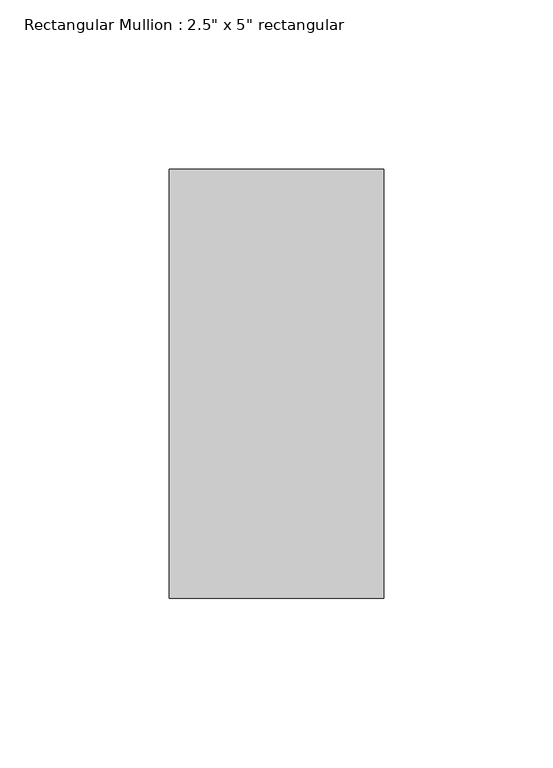
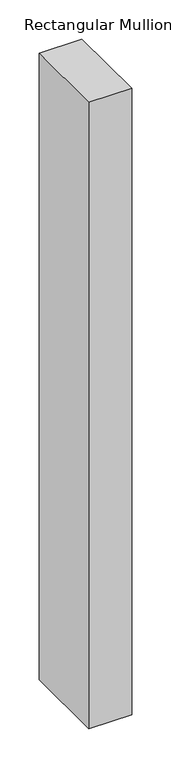
"""IFC4 building model written with IfcOpenShell, lengths in millimetres: member geometry."""

from ifc_helpers import new_model, si_unit, frame, origin, place, context, project, spatial, polyline, outline, extrude, source, transform, mapped, element, save


def member_6e6cbf30(model_context):
    return source(origin(), model_context, "Body", "SweptSolid", [
        extrude(outline(polyline([(0.0, 63.5), (0.0, -63.5), (-63.5, -63.5), (-63.5, 63.5), (0.0, 63.5)])), frame((0.0, 0.0, -979.7309713), z_axis=(0.0, 0.0, 1.0), x_axis=(1.0, 0.0, 0.0)), (0.0, 0.0, 1.0), 979.7309713),
    ])


if __name__ == "__main__":
    model = new_model("IFC4")
    model_context = context("Model", 3, world=origin())
    ifc_project = project(units=[si_unit("LENGTHUNIT", "METRE", prefix="MILLI")], contexts=[model_context])
    site = spatial("IfcSite", under=ifc_project)
    building = spatial("IfcBuilding", under=site)
    placement = place(None, origin())
    member_shape = member_6e6cbf30(model_context)
    element("IfcMember", 1, ObjectType="Rectangular Mullion : 2.5\" x 5\" rectangular", at=placement, inside=building, context=model_context, shape_type="MappedRepresentation", body=[
        mapped(member_shape, transform((0.0, 0.0, 0.0), x_axis=(1.0, 0.0, 0.0), y_axis=(0.0, 1.0, 0.0), z_axis=(0.0, 0.0, 1.0))),
    ])
    save(model, "model.ifc")

# Revit data of these elements
# Type "Rectangular Mullion : 2.5\" x 5\" rectangular"
#   built-in parameter 1007304 = 0.416667 (stored number, unit not read)
#   built-in parameter 1007301 = 0.104167 (stored number, unit not read)
#   built-in parameter 1007300 = 0.104167 (stored number, unit not read)
# Element 1 (IfcMember, "Rectangular Mullion : 2.5\" x 5\" rectangular")
#   Materials on its faces: "Aluminum"
# Materials
#   "Aluminum": class "Metal", colour RGB 247 247 247, transparency 0, Description = "Aluminum 6061", Cost = 0
